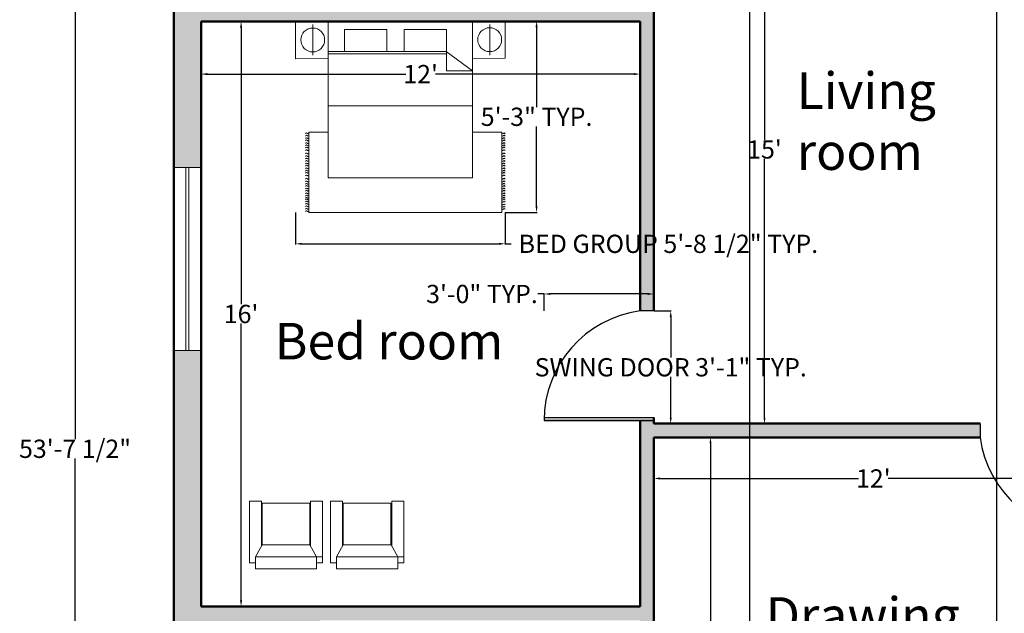
# Model space of a CAD drawing. Units: inches. Extents: x 2436 to 2989, y 5527 to 6207.
# Tile 2 of 5: x 2436 to 2759, y 5794 to 5989. Entities that reach past the tile are written whole.
import ezdxf

# ---------------------------------------------------------------- set-up
doc = ezdxf.new("R2010")
doc.units = ezdxf.units.IN
doc.header["$MEASUREMENT"] = 0
for name, color, linetype, lineweight in [('A-ANNO-DIMS', 2, 'Continuous', 18), ('A-AREA-IDEN', 7, 'Continuous', 25), ('A-DOOR', 3, 'Continuous', 25), ('A-FURN', 8, 'Continuous', 18), ('A-GLAZ', 4, 'Continuous', 18), ('A-WALL', 7, 'Continuous', 50), ('A-WALL-PATT', 252, 'Continuous', 13)]:
    doc.layers.add(name, color=color, linetype=linetype, lineweight=lineweight)
doc.styles.get("Standard").update_dxf_attribs({"font": 'arial.ttf'})
doc.dimstyles.get("Standard").update_dxf_attribs({"dimtxt": 6, "dimasz": 2, "dimexe": 0.18, "dimexo": 0.0625, "dimgap": 0.09, "dimtad": 0, "dimtih": 1, "dimtoh": 1, "dimdec": 0, "dimzin": 0, "dimdsep": 46, "dimlunit": 3, "dimtxsty": 'Standard', "dimcen": 0.09, "dimadec": 0, "dimazin": 0, "dimtfac": 1, "dimtdec": 0, "dimtofl": 0, "dimtmove": 0, "dimatfit": 3, "dimfxl": 1, "dimtolj": 1, "dimtzin": 0, "dimarcsym": 0})

# ---------------------------------------------------------------- blocks, each defined once
blk = doc.blocks.new('*D7')
at = {"layer": 'A-ANNO-DIMS', "color": 0, "lineweight": -2, "transparency": 16777216}
for p, q in [((2495.45, 5988.73), (2508.69, 5988.73)), ((2508.51, 5986.73), (2508.51, 5895.89)), ((2508.51, 5798.73), (2508.51, 5889.58)), ((2495.45, 5796.73), (2508.69, 5796.73))]:
    blk.add_line(p, q, dxfattribs=at)
at = {"layer": 'A-ANNO-DIMS', "color": 0, "transparency": 16777216}
for points in [[(2508.17, 5986.73), (2508.84, 5986.73), (2508.51, 5988.73)], [(2508.17, 5798.73), (2508.84, 5798.73), (2508.51, 5796.73)]]:
    blk.add_solid(points, dxfattribs=at)
at = {"layer": 'Defpoints', "color": 0, "transparency": 16777216}
for p in [(2495.39, 5988.73), (2495.39, 5796.73), (2508.51, 5796.73)]:
    blk.add_point(p, dxfattribs=at)
at = {"layer": 'A-ANNO-DIMS', "color": 0, "transparency": 16777216, "insert": (2508.51, 5892.73), "char_height": 6, "attachment_point": 5}
blk.add_mtext("\\A1;16'", dxfattribs=at)
blk = doc.blocks.new('*D8')
at = {"layer": 'A-ANNO-DIMS', "color": 0, "lineweight": -2, "transparency": 16777216}
for p, q in [((2495.39, 5988.67), (2495.39, 5971.26)), ((2639.39, 5988.67), (2639.39, 5971.26)), ((2497.39, 5971.44), (2562.49, 5971.44)), ((2637.39, 5971.44), (2572.29, 5971.44))]:
    blk.add_line(p, q, dxfattribs=at)
at = {"layer": 'A-ANNO-DIMS', "color": 0, "transparency": 16777216}
for points in [[(2497.39, 5971.78), (2497.39, 5971.11), (2495.39, 5971.44)], [(2637.39, 5971.78), (2637.39, 5971.11), (2639.39, 5971.44)]]:
    blk.add_solid(points, dxfattribs=at)
at = {"layer": 'Defpoints', "color": 0, "transparency": 16777216}
for p in [(2495.39, 5988.73), (2639.39, 5988.73), (2639.39, 5971.44)]:
    blk.add_point(p, dxfattribs=at)
at = {"layer": 'A-ANNO-DIMS', "color": 0, "transparency": 16777216, "insert": (2567.39, 5971.44), "char_height": 6, "attachment_point": 5}
blk.add_mtext("\\A1;12'", dxfattribs=at)
blk = doc.blocks.new('*D13')
at = {"layer": 'A-ANNO-DIMS', "color": 0, "lineweight": -2, "transparency": 16777216}
for p, q in [((2643.95, 5852.23), (2662.66, 5852.23)), ((2662.48, 5850.23), (2662.48, 5777.39)), ((2662.48, 5698.23), (2662.48, 5771.08)), ((2643.95, 5696.23), (2662.66, 5696.23))]:
    blk.add_line(p, q, dxfattribs=at)
at = {"layer": 'A-ANNO-DIMS', "color": 0, "transparency": 16777216}
for points in [[(2662.15, 5850.23), (2662.81, 5850.23), (2662.48, 5852.23)], [(2662.15, 5698.23), (2662.81, 5698.23), (2662.48, 5696.23)]]:
    blk.add_solid(points, dxfattribs=at)
at = {"layer": 'Defpoints', "color": 0, "transparency": 16777216}
for p in [(2643.89, 5852.23), (2643.89, 5696.23), (2662.48, 5696.23)]:
    blk.add_point(p, dxfattribs=at)
at = {"layer": 'A-ANNO-DIMS', "color": 0, "transparency": 16777216, "insert": (2662.48, 5774.23), "char_height": 6, "attachment_point": 5}
blk.add_mtext("\\A1;13'", dxfattribs=at)
blk = doc.blocks.new('*D14')
at = {"layer": 'A-ANNO-DIMS', "color": 0, "lineweight": -2, "transparency": 16777216}
for p, q in [((2643.89, 5852.17), (2643.89, 5838.55)), ((2787.89, 5852.17), (2787.89, 5838.55)), ((2645.89, 5838.73), (2710.99, 5838.73)), ((2785.89, 5838.73), (2720.79, 5838.73))]:
    blk.add_line(p, q, dxfattribs=at)
at = {"layer": 'A-ANNO-DIMS', "color": 0, "transparency": 16777216}
for points in [[(2645.89, 5839.07), (2645.89, 5838.4), (2643.89, 5838.73)], [(2785.89, 5839.07), (2785.89, 5838.4), (2787.89, 5838.73)]]:
    blk.add_solid(points, dxfattribs=at)
at = {"layer": 'Defpoints', "color": 0, "transparency": 16777216}
for p in [(2643.89, 5852.23), (2787.89, 5852.23), (2787.89, 5838.73)]:
    blk.add_point(p, dxfattribs=at)
at = {"layer": 'A-ANNO-DIMS', "color": 0, "transparency": 16777216, "insert": (2715.89, 5838.73), "char_height": 6, "attachment_point": 5}
blk.add_mtext("\\A1;12'", dxfattribs=at)
blk = doc.blocks.new('*D19')
at = {"layer": 'A-ANNO-DIMS', "color": 0, "lineweight": -2, "transparency": 16777216}
for p, q in [((2667.17, 6036.73), (2680.37, 6036.73)), ((2680.19, 6034.73), (2680.19, 5949.89)), ((2680.19, 5858.73), (2680.19, 5943.58)), ((2667.17, 5856.73), (2680.37, 5856.73))]:
    blk.add_line(p, q, dxfattribs=at)
at = {"layer": 'A-ANNO-DIMS', "color": 0, "transparency": 16777216}
for points in [[(2679.86, 6034.73), (2680.52, 6034.73), (2680.19, 6036.73)], [(2679.86, 5858.73), (2680.52, 5858.73), (2680.19, 5856.73)]]:
    blk.add_solid(points, dxfattribs=at)
at = {"layer": 'Defpoints', "color": 0, "transparency": 16777216}
for p in [(2667.11, 6036.73), (2667.11, 5856.73), (2680.19, 5856.73)]:
    blk.add_point(p, dxfattribs=at)
at = {"layer": 'A-ANNO-DIMS', "color": 0, "transparency": 16777216, "insert": (2680.19, 5946.73), "char_height": 6, "attachment_point": 5}
blk.add_mtext("\\A1;15'", dxfattribs=at)
blk = doc.blocks.new('BED-WITH-NIGHTSTANDS')
for p, q in [((5.6, 61.62), (5.6, 51.56)), ((63.65, 61.72), (63.65, 51.66)), ((49.39, 52.82), (10.63, 52.82)), ((49.44, 52), (10.63, 52)), ((49.39, 52.82), (58, 46.47)), ((49.44, 52.82), (49.44, 46.47)), ((49.44, 46.47), (58, 46.47)), ((58.05, 34.96), (10.63, 34.96)), ((4.35, 0), (4.35, 26.37)), ((4.35, 26.37), (10.65, 26.37)), ((58.05, 26.37), (67.59, 26.37)), ((67.59, 26.37), (67.59, 0)), ((4.35, 0), (67.59, 0))]:
    blk.add_line(p, q)
for points in [[(0, 50.39), (10.63, 50.5), (10.63, 62.68), (0, 62.58)], [(58.05, 62.68), (58.05, 11.37), (10.63, 11.37), (10.63, 62.68)], [(58.05, 50.5), (68.68, 50.6), (68.68, 62.78), (58.05, 62.68)], [(29.88, 59.98), (29.88, 52.82), (15.98, 52.82), (15.98, 59.98)], [(49.44, 59.98), (49.44, 52.82), (35.55, 52.82), (35.55, 59.98)]]:
    blk.add_lwpolyline(points, close=True)
for centre in [(5.6, 56.59), (63.65, 56.69)]:
    blk.add_circle(centre, 3.92)
for points, knots in [([(3.23, 25.84), (3.32, 25.96), (3.52, 26.2), (3.86, 25.96), (4.14, 25.78), (4.29, 25.89), (4.35, 25.94)], [0, 0, 0, 0, 0.400747, 0.791423, 1.067667, 1.29709, 1.29709, 1.29709, 1.29709]), ([(68.71, 25.84), (68.61, 25.96), (68.42, 26.2), (68.08, 25.96), (67.8, 25.78), (67.65, 25.89), (67.58, 25.94)], [0, 0, 0, 0, 0.400747, 0.791423, 1.067667, 1.29709, 1.29709, 1.29709, 1.29709]), ([(3.23, 25.06), (3.32, 25.18), (3.52, 25.42), (3.86, 25.18), (4.14, 25.01), (4.29, 25.11), (4.35, 25.16)], [0, 0, 0, 0, 0.400747, 0.791423, 1.067667, 1.29709, 1.29709, 1.29709, 1.29709]), ([(3.23, 24.24), (3.32, 24.36), (3.52, 24.6), (3.86, 24.36), (4.14, 24.19), (4.29, 24.3), (4.35, 24.34)], [0, 0, 0, 0, 0.400747, 0.791423, 1.067667, 1.29709, 1.29709, 1.29709, 1.29709]), ([(3.23, 23.51), (3.32, 23.63), (3.52, 23.87), (3.86, 23.63), (4.14, 23.46), (4.29, 23.57), (4.35, 23.62)], [0, 0, 0, 0, 0.400747, 0.791423, 1.067667, 1.29709, 1.29709, 1.29709, 1.29709]), ([(3.23, 22.63), (3.32, 22.75), (3.52, 22.99), (3.86, 22.75), (4.14, 22.58), (4.29, 22.69), (4.35, 22.73)], [0, 0, 0, 0, 0.400747, 0.791423, 1.067667, 1.29709, 1.29709, 1.29709, 1.29709]), ([(68.71, 25.06), (68.61, 25.18), (68.42, 25.42), (68.08, 25.18), (67.8, 25.01), (67.65, 25.11), (67.58, 25.16)], [0, 0, 0, 0, 0.400747, 0.791423, 1.067667, 1.29709, 1.29709, 1.29709, 1.29709]), ([(68.71, 24.24), (68.61, 24.36), (68.42, 24.6), (68.08, 24.36), (67.8, 24.19), (67.65, 24.3), (67.58, 24.34)], [0, 0, 0, 0, 0.400747, 0.791423, 1.067667, 1.29709, 1.29709, 1.29709, 1.29709]), ([(68.71, 23.51), (68.61, 23.63), (68.42, 23.87), (68.08, 23.63), (67.8, 23.46), (67.65, 23.57), (67.58, 23.62)], [0, 0, 0, 0, 0.400747, 0.791423, 1.067667, 1.29709, 1.29709, 1.29709, 1.29709]), ([(68.71, 22.63), (68.61, 22.75), (68.42, 22.99), (68.08, 22.75), (67.8, 22.58), (67.65, 22.69), (67.58, 22.73)], [0, 0, 0, 0, 0.400747, 0.791423, 1.067667, 1.29709, 1.29709, 1.29709, 1.29709]), ([(3.23, 21.88), (3.32, 22), (3.52, 22.24), (3.86, 22), (4.14, 21.83), (4.29, 21.93), (4.35, 21.98)], [0, 0, 0, 0, 0.400747, 0.791423, 1.067667, 1.29709, 1.29709, 1.29709, 1.29709]), ([(3.23, 21.15), (3.32, 21.27), (3.52, 21.51), (3.86, 21.27), (4.14, 21.1), (4.29, 21.21), (4.35, 21.25)], [0, 0, 0, 0, 0.400747, 0.791423, 1.067667, 1.29709, 1.29709, 1.29709, 1.29709]), ([(3.23, 20.27), (3.32, 20.39), (3.52, 20.63), (3.86, 20.39), (4.14, 20.22), (4.29, 20.32), (4.35, 20.37)], [0, 0, 0, 0, 0.400747, 0.791423, 1.067667, 1.29709, 1.29709, 1.29709, 1.29709]), ([(3.23, 19.23), (3.32, 19.35), (3.52, 19.59), (3.86, 19.35), (4.14, 19.18), (4.29, 19.29), (4.35, 19.33)], [0, 0, 0, 0, 0.400747, 0.791423, 1.067667, 1.29709, 1.29709, 1.29709, 1.29709]), ([(68.71, 21.88), (68.61, 22), (68.42, 22.24), (68.08, 22), (67.8, 21.83), (67.65, 21.93), (67.58, 21.98)], [0, 0, 0, 0, 0.400747, 0.791423, 1.067667, 1.29709, 1.29709, 1.29709, 1.29709]), ([(68.71, 21.15), (68.61, 21.27), (68.42, 21.51), (68.08, 21.27), (67.8, 21.1), (67.65, 21.21), (67.58, 21.25)], [0, 0, 0, 0, 0.400747, 0.791423, 1.067667, 1.29709, 1.29709, 1.29709, 1.29709]), ([(68.71, 20.27), (68.61, 20.39), (68.42, 20.63), (68.08, 20.39), (67.8, 20.22), (67.65, 20.32), (67.58, 20.37)], [0, 0, 0, 0, 0.400747, 0.791423, 1.067667, 1.29709, 1.29709, 1.29709, 1.29709]), ([(68.71, 19.23), (68.61, 19.35), (68.42, 19.59), (68.08, 19.35), (67.8, 19.18), (67.65, 19.29), (67.58, 19.33)], [0, 0, 0, 0, 0.400747, 0.791423, 1.067667, 1.29709, 1.29709, 1.29709, 1.29709]), ([(3.23, 18.35), (3.32, 18.47), (3.52, 18.71), (3.86, 18.47), (4.14, 18.3), (4.29, 18.4), (4.35, 18.45)], [0, 0, 0, 0, 0.400747, 0.791423, 1.067667, 1.29709, 1.29709, 1.29709, 1.29709]), ([(3.23, 17.53), (3.32, 17.65), (3.52, 17.89), (3.86, 17.65), (4.14, 17.48), (4.29, 17.59), (4.35, 17.64)], [0, 0, 0, 0, 0.400747, 0.791423, 1.067667, 1.29709, 1.29709, 1.29709, 1.29709]), ([(3.23, 16.76), (3.32, 16.88), (3.52, 17.12), (3.86, 16.88), (4.14, 16.71), (4.29, 16.81), (4.35, 16.86)], [0, 0, 0, 0, 0.400747, 0.791423, 1.067667, 1.29709, 1.29709, 1.29709, 1.29709]), ([(3.23, 15.94), (3.32, 16.06), (3.52, 16.3), (3.86, 16.06), (4.14, 15.89), (4.29, 16), (4.35, 16.04)], [0, 0, 0, 0, 0.400747, 0.791423, 1.067667, 1.29709, 1.29709, 1.29709, 1.29709]), ([(68.71, 18.35), (68.61, 18.47), (68.42, 18.71), (68.08, 18.47), (67.8, 18.3), (67.65, 18.4), (67.58, 18.45)], [0, 0, 0, 0, 0.400747, 0.791423, 1.067667, 1.29709, 1.29709, 1.29709, 1.29709]), ([(68.71, 17.53), (68.61, 17.65), (68.42, 17.89), (68.08, 17.65), (67.8, 17.48), (67.65, 17.59), (67.58, 17.64)], [0, 0, 0, 0, 0.400747, 0.791423, 1.067667, 1.29709, 1.29709, 1.29709, 1.29709]), ([(68.71, 16.76), (68.61, 16.88), (68.42, 17.12), (68.08, 16.88), (67.8, 16.71), (67.65, 16.81), (67.58, 16.86)], [0, 0, 0, 0, 0.400747, 0.791423, 1.067667, 1.29709, 1.29709, 1.29709, 1.29709]), ([(68.71, 15.94), (68.61, 16.06), (68.42, 16.3), (68.08, 16.06), (67.8, 15.89), (67.65, 16), (67.58, 16.04)], [0, 0, 0, 0, 0.400747, 0.791423, 1.067667, 1.29709, 1.29709, 1.29709, 1.29709]), ([(3.23, 15.21), (3.32, 15.33), (3.52, 15.57), (3.86, 15.33), (4.14, 15.16), (4.29, 15.27), (4.35, 15.32)], [0, 0, 0, 0, 0.400747, 0.791423, 1.067667, 1.29709, 1.29709, 1.29709, 1.29709]), ([(3.23, 14.33), (3.32, 14.45), (3.52, 14.69), (3.86, 14.45), (4.14, 14.28), (4.29, 14.39), (4.35, 14.43)], [0, 0, 0, 0, 0.400747, 0.791423, 1.067667, 1.29709, 1.29709, 1.29709, 1.29709]), ([(3.23, 13.58), (3.32, 13.7), (3.52, 13.94), (3.86, 13.7), (4.14, 13.53), (4.29, 13.63), (4.35, 13.68)], [0, 0, 0, 0, 0.400747, 0.791423, 1.067667, 1.29709, 1.29709, 1.29709, 1.29709]), ([(3.23, 12.85), (3.32, 12.97), (3.52, 13.21), (3.86, 12.97), (4.14, 12.8), (4.29, 12.9), (4.35, 12.95)], [0, 0, 0, 0, 0.400747, 0.791423, 1.067667, 1.29709, 1.29709, 1.29709, 1.29709]), ([(68.71, 15.21), (68.61, 15.33), (68.42, 15.57), (68.08, 15.33), (67.8, 15.16), (67.65, 15.27), (67.58, 15.32)], [0, 0, 0, 0, 0.400747, 0.791423, 1.067667, 1.29709, 1.29709, 1.29709, 1.29709]), ([(68.71, 14.33), (68.61, 14.45), (68.42, 14.69), (68.08, 14.45), (67.8, 14.28), (67.65, 14.39), (67.58, 14.43)], [0, 0, 0, 0, 0.400747, 0.791423, 1.067667, 1.29709, 1.29709, 1.29709, 1.29709]), ([(68.71, 13.58), (68.61, 13.7), (68.42, 13.94), (68.08, 13.7), (67.8, 13.53), (67.65, 13.63), (67.58, 13.68)], [0, 0, 0, 0, 0.400747, 0.791423, 1.067667, 1.29709, 1.29709, 1.29709, 1.29709]), ([(68.71, 12.85), (68.61, 12.97), (68.42, 13.21), (68.08, 12.97), (67.8, 12.8), (67.65, 12.9), (67.58, 12.95)], [0, 0, 0, 0, 0.400747, 0.791423, 1.067667, 1.29709, 1.29709, 1.29709, 1.29709]), ([(3.23, 11.97), (3.32, 12.09), (3.52, 12.33), (3.86, 12.09), (4.14, 11.92), (4.29, 12.02), (4.35, 12.07)], [0, 0, 0, 0, 0.400747, 0.791423, 1.067667, 1.29709, 1.29709, 1.29709, 1.29709]), ([(3.23, 10.93), (3.32, 11.05), (3.52, 11.29), (3.86, 11.05), (4.14, 10.88), (4.29, 10.99), (4.35, 11.03)], [0, 0, 0, 0, 0.400747, 0.791423, 1.067667, 1.29709, 1.29709, 1.29709, 1.29709]), ([(3.23, 10.05), (3.32, 10.17), (3.52, 10.41), (3.86, 10.17), (4.14, 10), (4.29, 10.1), (4.35, 10.15)], [0, 0, 0, 0, 0.400747, 0.791423, 1.067667, 1.29709, 1.29709, 1.29709, 1.29709]), ([(68.71, 11.97), (68.61, 12.09), (68.42, 12.33), (68.08, 12.09), (67.8, 11.92), (67.65, 12.02), (67.58, 12.07)], [0, 0, 0, 0, 0.400747, 0.791423, 1.067667, 1.29709, 1.29709, 1.29709, 1.29709]), ([(68.71, 10.93), (68.61, 11.05), (68.42, 11.29), (68.08, 11.05), (67.8, 10.88), (67.65, 10.99), (67.58, 11.03)], [0, 0, 0, 0, 0.400747, 0.791423, 1.067667, 1.29709, 1.29709, 1.29709, 1.29709]), ([(68.71, 10.05), (68.61, 10.17), (68.42, 10.41), (68.08, 10.17), (67.8, 10), (67.65, 10.1), (67.58, 10.15)], [0, 0, 0, 0, 0.400747, 0.791423, 1.067667, 1.29709, 1.29709, 1.29709, 1.29709]), ([(3.23, 9.23), (3.32, 9.35), (3.52, 9.59), (3.86, 9.35), (4.14, 9.18), (4.29, 9.29), (4.35, 9.34)], [0, 0, 0, 0, 0.400747, 0.791423, 1.067667, 1.29709, 1.29709, 1.29709, 1.29709]), ([(3.23, 8.54), (3.32, 8.66), (3.52, 8.9), (3.86, 8.66), (4.14, 8.49), (4.29, 8.6), (4.35, 8.65)], [0, 0, 0, 0, 0.400747, 0.791423, 1.067667, 1.29709, 1.29709, 1.29709, 1.29709]), ([(3.23, 7.73), (3.32, 7.85), (3.52, 8.09), (3.86, 7.85), (4.14, 7.68), (4.29, 7.78), (4.35, 7.83)], [0, 0, 0, 0, 0.400747, 0.791423, 1.067667, 1.29709, 1.29709, 1.29709, 1.29709]), ([(3.23, 7), (3.32, 7.12), (3.52, 7.36), (3.86, 7.12), (4.14, 6.95), (4.29, 7.05), (4.35, 7.1)], [0, 0, 0, 0, 0.400747, 0.791423, 1.067667, 1.29709, 1.29709, 1.29709, 1.29709]), ([(68.71, 9.23), (68.61, 9.35), (68.42, 9.59), (68.08, 9.35), (67.8, 9.18), (67.65, 9.29), (67.58, 9.34)], [0, 0, 0, 0, 0.400747, 0.791423, 1.067667, 1.29709, 1.29709, 1.29709, 1.29709]), ([(68.71, 8.54), (68.61, 8.66), (68.42, 8.9), (68.08, 8.66), (67.8, 8.49), (67.65, 8.6), (67.58, 8.65)], [0, 0, 0, 0, 0.400747, 0.791423, 1.067667, 1.29709, 1.29709, 1.29709, 1.29709]), ([(68.71, 7.73), (68.61, 7.85), (68.42, 8.09), (68.08, 7.85), (67.8, 7.68), (67.65, 7.78), (67.58, 7.83)], [0, 0, 0, 0, 0.400747, 0.791423, 1.067667, 1.29709, 1.29709, 1.29709, 1.29709]), ([(68.71, 7), (68.61, 7.12), (68.42, 7.36), (68.08, 7.12), (67.8, 6.95), (67.65, 7.05), (67.58, 7.1)], [0, 0, 0, 0, 0.400747, 0.791423, 1.067667, 1.29709, 1.29709, 1.29709, 1.29709]), ([(3.23, 6.12), (3.32, 6.24), (3.52, 6.48), (3.86, 6.24), (4.14, 6.07), (4.29, 6.17), (4.35, 6.22)], [0, 0, 0, 0, 0.400747, 0.791423, 1.067667, 1.29709, 1.29709, 1.29709, 1.29709]), ([(3.23, 5.36), (3.32, 5.49), (3.52, 5.73), (3.86, 5.49), (4.14, 5.31), (4.29, 5.42), (4.35, 5.47)], [0, 0, 0, 0, 0.400747, 0.791423, 1.067667, 1.29709, 1.29709, 1.29709, 1.29709]), ([(3.23, 4.64), (3.32, 4.76), (3.52, 5), (3.86, 4.76), (4.14, 4.59), (4.29, 4.69), (4.35, 4.74)], [0, 0, 0, 0, 0.400747, 0.791423, 1.067667, 1.29709, 1.29709, 1.29709, 1.29709]), ([(3.23, 4.13), (3.32, 4.25), (3.52, 4.49), (3.86, 4.25), (4.14, 4.08), (4.29, 4.18), (4.35, 4.23)], [0, 0, 0, 0, 0.400747, 0.791423, 1.067667, 1.29709, 1.29709, 1.29709, 1.29709]), ([(3.23, 3.44), (3.32, 3.56), (3.52, 3.8), (3.86, 3.56), (4.14, 3.39), (4.29, 3.49), (4.35, 3.54)], [0, 0, 0, 0, 0.400747, 0.791423, 1.067667, 1.29709, 1.29709, 1.29709, 1.29709]), ([(68.71, 6.12), (68.61, 6.24), (68.42, 6.48), (68.08, 6.24), (67.8, 6.07), (67.65, 6.17), (67.58, 6.22)], [0, 0, 0, 0, 0.400747, 0.791423, 1.067667, 1.29709, 1.29709, 1.29709, 1.29709]), ([(68.71, 5.36), (68.61, 5.49), (68.42, 5.73), (68.08, 5.49), (67.8, 5.31), (67.65, 5.42), (67.58, 5.47)], [0, 0, 0, 0, 0.400747, 0.791423, 1.067667, 1.29709, 1.29709, 1.29709, 1.29709]), ([(68.71, 4.64), (68.61, 4.76), (68.42, 5), (68.08, 4.76), (67.8, 4.59), (67.66, 4.69), (67.59, 4.73)], [0, 0, 0, 0, 0.400747, 0.791423, 1.067667, 1.283686, 1.283686, 1.283686, 1.283686]), ([(68.72, 4.07), (68.62, 4.19), (68.43, 4.43), (68.09, 4.19), (67.81, 4.01), (67.66, 4.12), (67.59, 4.17)], [0, 0, 0, 0, 0.400747, 0.791423, 1.067667, 1.29709, 1.29709, 1.29709, 1.29709]), ([(68.72, 3.34), (68.62, 3.46), (68.43, 3.7), (68.09, 3.46), (67.81, 3.29), (67.66, 3.39), (67.59, 3.44)], [0, 0, 0, 0, 0.400747, 0.791423, 1.067667, 1.29709, 1.29709, 1.29709, 1.29709]), ([(3.23, 2.67), (3.32, 2.79), (3.52, 3.03), (3.86, 2.79), (4.14, 2.62), (4.29, 2.73), (4.35, 2.78)], [0, 0, 0, 0, 0.400747, 0.791423, 1.067667, 1.29709, 1.29709, 1.29709, 1.29709]), ([(3.23, 1.86), (3.32, 1.98), (3.52, 2.22), (3.86, 1.98), (4.14, 1.81), (4.29, 1.92), (4.35, 1.97)], [0, 0, 0, 0, 0.400747, 0.791423, 1.067667, 1.29709, 1.29709, 1.29709, 1.29709]), ([(3.23, 1.05), (3.32, 1.17), (3.52, 1.41), (3.86, 1.17), (4.14, 1), (4.29, 1.11), (4.35, 1.15)], [0, 0, 0, 0, 0.400747, 0.791423, 1.067667, 1.29709, 1.29709, 1.29709, 1.29709]), ([(3.23, 0.28), (3.32, 0.4), (3.52, 0.64), (3.86, 0.4), (4.14, 0.22), (4.29, 0.33), (4.35, 0.38)], [0, 0, 0, 0, 0.400747, 0.791423, 1.067667, 1.29709, 1.29709, 1.29709, 1.29709]), ([(68.72, 2.46), (68.62, 2.58), (68.43, 2.82), (68.09, 2.58), (67.81, 2.4), (67.66, 2.51), (67.59, 2.56)], [0, 0, 0, 0, 0.400747, 0.791423, 1.067667, 1.29709, 1.29709, 1.29709, 1.29709]), ([(68.72, 1.7), (68.62, 1.82), (68.43, 2.06), (68.09, 1.82), (67.81, 1.65), (67.66, 1.76), (67.59, 1.81)], [0, 0, 0, 0, 0.400747, 0.791423, 1.067667, 1.29709, 1.29709, 1.29709, 1.29709]), ([(68.72, 0.98), (68.62, 1.1), (68.43, 1.34), (68.09, 1.1), (67.81, 0.93), (67.67, 1.03), (67.6, 1.07)], [0, 0, 0, 0, 0.400747, 0.791423, 1.067667, 1.283686, 1.283686, 1.283686, 1.283686])]:
    blk.add_open_spline(points, degree=3, knots=knots)
blk = doc.blocks.new('CHAIR-ARM')
for p, q in [((0, 1.96), (0, 22.23)), ((3.92, 22.23), (0, 22.23)), ((3.92, 7.54), (3.92, 22.23)), ((19.74, 21.58), (19.74, 7.85)), ((20.05, 7.41), (20.05, 22.23)), ((20.05, 22.23), (23.98, 22.23)), ((23.98, 1.96), (23.98, 22.23)), ((1.96, 3.92), (4.17, 7.85)), ((19.81, 7.85), (22.01, 3.92)), ((1.96, 3.92), (23.98, 3.92)), ((1.96, 3.92), (1.96, 0)), ((22.01, 3.92), (22.01, 0)), ((0, 1.96), (1.96, 1.96)), ((1.96, 0), (22.01, 0)), ((22.01, 1.96), (23.98, 1.96))]:
    blk.add_line(p, q)
blk.add_lwpolyline([(19.74, 21.58), (4.17, 21.58), (4.17, 7.85), (19.81, 7.85)])
blk = doc.blocks.new('WINDOW-60IN')
for p, q in [((0, 9), (0, 0)), ((60, 9), (0, 9)), ((60, 0), (60, 9)), ((60, 5), (0, 5)), ((0, 4), (60, 4)), ((0, 0), (60, 0))]:
    blk.add_line(p, q)
blk = doc.blocks.new('DOOR-SWING-36IN')
for p, q in [((1, 0), (1, 36)), ((1, 36), (1, 0)), ((2, 36), (2, 0)), ((37, 0), (37, 4.5)), ((0, 0), (1, 0)), ((1, 0), (2, 0))]:
    blk.add_line(p, q)
blk.add_arc((1, -0.32), 36.32, 7.6281, 90)
blk = doc.blocks.new('*D34')
at = {"layer": 'A-ANNO-DIMS', "color": 0, "lineweight": -2, "transparency": 16777216}
for p, q in [((2553.14, 6000.14), (2553.14, 5996.42)), ((2577.11, 6000.14), (2577.11, 5996.42)), ((2555.14, 5996.6), (2575.11, 5996.6)), ((2577.11, 5996.6), (2579.11, 5996.6))]:
    blk.add_line(p, q, dxfattribs=at)
at = {"layer": 'A-ANNO-DIMS', "color": 0, "transparency": 16777216}
for points in [[(2555.14, 5996.94), (2555.14, 5996.27), (2553.14, 5996.6)], [(2575.11, 5996.94), (2575.11, 5996.27), (2577.11, 5996.6)]]:
    blk.add_solid(points, dxfattribs=at)
at = {"layer": 'Defpoints', "color": 0, "transparency": 16777216}
for p in [(2553.14, 6000.2), (2577.11, 6000.2), (2577.11, 5996.6)]:
    blk.add_point(p, dxfattribs=at)
at = {"layer": 'A-ANNO-DIMS', "color": 0, "transparency": 16777216, "insert": (2621.18, 5996.6), "char_height": 6, "attachment_point": 5}
blk.add_mtext('\\A1;ARMCHAIR 2\'-0" TYP.', dxfattribs=at)
blk = doc.blocks.new('*D36')
at = {"layer": 'A-ANNO-DIMS', "color": 0, "lineweight": -2, "transparency": 16777216}
for p, q in [((2526.4, 5925.99), (2526.4, 5915.56)), ((2595.12, 5925.99), (2595.12, 5915.56)), ((2528.4, 5915.74), (2593.12, 5915.74)), ((2595.12, 5915.74), (2597.12, 5915.74))]:
    blk.add_line(p, q, dxfattribs=at)
at = {"layer": 'A-ANNO-DIMS', "color": 0, "transparency": 16777216}
for points in [[(2528.4, 5916.08), (2528.4, 5915.41), (2526.4, 5915.74)], [(2593.12, 5916.08), (2593.12, 5915.41), (2595.12, 5915.74)]]:
    blk.add_solid(points, dxfattribs=at)
at = {"layer": 'Defpoints', "color": 0, "transparency": 16777216}
for p in [(2526.4, 5926.05), (2595.12, 5926.05), (2595.12, 5915.74)]:
    blk.add_point(p, dxfattribs=at)
at = {"layer": 'A-ANNO-DIMS', "color": 0, "transparency": 16777216, "insert": (2648.67, 5915.74), "char_height": 6, "attachment_point": 5}
blk.add_mtext('\\A1;BED GROUP 5\'-8 1/2" TYP.', dxfattribs=at)
blk = doc.blocks.new('*D37')
at = {"layer": 'A-ANNO-DIMS', "color": 0, "lineweight": -2, "transparency": 16777216}
for p, q in [((2595.18, 5988.83), (2605.61, 5988.83)), ((2605.43, 5986.83), (2605.43, 5960.6)), ((2605.43, 5928.05), (2605.43, 5954.29)), ((2595.18, 5926.05), (2605.61, 5926.05))]:
    blk.add_line(p, q, dxfattribs=at)
at = {"layer": 'A-ANNO-DIMS', "color": 0, "transparency": 16777216}
for points in [[(2605.09, 5986.83), (2605.76, 5986.83), (2605.43, 5988.83)], [(2605.09, 5928.05), (2605.76, 5928.05), (2605.43, 5926.05)]]:
    blk.add_solid(points, dxfattribs=at)
at = {"layer": 'Defpoints', "color": 0, "transparency": 16777216}
for p in [(2595.12, 5988.83), (2605.43, 5988.83), (2595.12, 5926.05)]:
    blk.add_point(p, dxfattribs=at)
at = {"layer": 'A-ANNO-DIMS', "color": 0, "transparency": 16777216, "insert": (2605.43, 5957.44), "char_height": 6, "attachment_point": 5}
blk.add_mtext('\\A1;5\'-3" TYP.', dxfattribs=at)
blk = doc.blocks.new('*D40')
at = {"layer": 'A-ANNO-DIMS', "color": 0, "lineweight": -2, "transparency": 16777216}
for p, q in [((2643.95, 5893.73), (2649.62, 5893.73)), ((2649.44, 5891.73), (2649.44, 5878.43)), ((2649.44, 5858.73), (2649.44, 5872.04)), ((2643.95, 5856.73), (2649.62, 5856.73))]:
    blk.add_line(p, q, dxfattribs=at)
at = {"layer": 'A-ANNO-DIMS', "color": 0, "transparency": 16777216}
for points in [[(2649.1, 5891.73), (2649.77, 5891.73), (2649.44, 5893.73)], [(2649.1, 5858.73), (2649.77, 5858.73), (2649.44, 5856.73)]]:
    blk.add_solid(points, dxfattribs=at)
at = {"layer": 'Defpoints', "color": 0, "transparency": 16777216}
for p in [(2643.89, 5893.73), (2649.44, 5893.73), (2643.89, 5856.73)]:
    blk.add_point(p, dxfattribs=at)
at = {"layer": 'A-ANNO-DIMS', "color": 0, "transparency": 16777216, "insert": (2649.44, 5875.23), "char_height": 6, "attachment_point": 5}
blk.add_mtext('\\A1;SWING DOOR 3\'-1" TYP.', dxfattribs=at)
blk = doc.blocks.new('*D41')
at = {"layer": 'A-ANNO-DIMS', "color": 0, "lineweight": -2, "transparency": 16777216}
for p, q in [((2607.89, 5899.28), (2605.89, 5899.28)), ((2607.89, 5893.79), (2607.89, 5899.46)), ((2641.89, 5899.28), (2609.89, 5899.28)), ((2643.89, 5893.79), (2643.89, 5899.46))]:
    blk.add_line(p, q, dxfattribs=at)
at = {"layer": 'A-ANNO-DIMS', "color": 0, "transparency": 16777216}
for points in [[(2609.89, 5899.62), (2609.89, 5898.95), (2607.89, 5899.28)], [(2641.89, 5899.62), (2641.89, 5898.95), (2643.89, 5899.28)]]:
    blk.add_solid(points, dxfattribs=at)
at = {"layer": 'Defpoints', "color": 0, "transparency": 16777216}
for p in [(2607.89, 5899.28), (2607.89, 5893.73), (2643.89, 5893.73)]:
    blk.add_point(p, dxfattribs=at)
at = {"layer": 'A-ANNO-DIMS', "color": 0, "transparency": 16777216, "insert": (2587.51, 5899.28), "char_height": 6, "attachment_point": 5}
blk.add_mtext('\\A1;3\'-0" TYP.', dxfattribs=at)
blk = doc.blocks.new('*D49')
at = {"layer": 'A-ANNO-DIMS', "color": 0, "lineweight": -2, "transparency": 16777216}
for p, q in [((2486.33, 6170.23), (2453.86, 6170.23)), ((2454.04, 6168.23), (2454.04, 5851.68)), ((2454.04, 5528.73), (2454.04, 5845.29)), ((2675.33, 5526.73), (2453.86, 5526.73))]:
    blk.add_line(p, q, dxfattribs=at)
at = {"layer": 'A-ANNO-DIMS', "color": 0, "transparency": 16777216}
for points in [[(2453.7, 6168.23), (2454.37, 6168.23), (2454.04, 6170.23)], [(2453.7, 5528.73), (2454.37, 5528.73), (2454.04, 5526.73)]]:
    blk.add_solid(points, dxfattribs=at)
at = {"layer": 'Defpoints', "color": 0, "transparency": 16777216}
for p in [(2486.39, 6170.23), (2454.04, 5526.73), (2675.39, 5526.73)]:
    blk.add_point(p, dxfattribs=at)
at = {"layer": 'A-ANNO-DIMS', "color": 0, "transparency": 16777216, "insert": (2454.04, 5848.48), "char_height": 6, "attachment_point": 5}
blk.add_mtext('\\A1;53\'-7 1/2"', dxfattribs=at)
blk = doc.blocks.new('*D51')
at = {"layer": 'A-ANNO-DIMS', "color": 0, "lineweight": -2, "transparency": 16777216}
for p, q in [((2675.39, 5526.79), (2675.39, 6202.76)), ((2677.39, 6202.58), (2707.81, 6202.58)), ((2754.39, 6202.58), (2723.97, 6202.58)), ((2756.39, 5526.79), (2756.39, 6202.76))]:
    blk.add_line(p, q, dxfattribs=at)
at = {"layer": 'A-ANNO-DIMS', "color": 0, "transparency": 16777216}
for points in [[(2677.39, 6202.92), (2677.39, 6202.25), (2675.39, 6202.58)], [(2754.39, 6202.92), (2754.39, 6202.25), (2756.39, 6202.58)]]:
    blk.add_solid(points, dxfattribs=at)
at = {"layer": 'Defpoints', "color": 0, "transparency": 16777216}
for p in [(2756.39, 6202.58), (2675.39, 5526.73), (2756.39, 5526.73)]:
    blk.add_point(p, dxfattribs=at)
at = {"layer": 'A-ANNO-DIMS', "color": 0, "transparency": 16777216, "insert": (2715.89, 6202.58), "char_height": 6, "attachment_point": 5}
blk.add_mtext('\\A1;6\'-9"', dxfattribs=at)
blk = doc.blocks.new('*D54')
at = {"layer": 'A-ANNO-DIMS', "color": 0, "lineweight": -2, "transparency": 16777216}
for p, q in [((2638.98, 6035.73), (2639.16, 6035.73)), ((2639.07, 6035.64), (2639.07, 6035.82)), ((2682.8, 5997.46), (2667.91, 6010.5)), ((2684.8, 5997.46), (2682.8, 5997.46))]:
    blk.add_line(p, q, dxfattribs=at)
at = {"layer": 'A-ANNO-DIMS', "color": 0, "transparency": 16777216}
blk.add_solid([(2668.13, 6010.75), (2667.69, 6010.25), (2666.4, 6011.81)], dxfattribs=at)
at = {"layer": 'Defpoints', "color": 0, "transparency": 16777216}
for p in [(2639.07, 6035.73), (2666.4, 6011.81)]:
    blk.add_point(p, dxfattribs=at)
at = {"layer": 'A-ANNO-DIMS', "color": 0, "transparency": 16777216, "insert": (2709.19, 5997.46), "char_height": 6, "attachment_point": 5}
blk.add_mtext('\\A1;6X R3\'-0 1/2"', dxfattribs=at)

msp = doc.modelspace()

# ---------------------------------------------------------------- hatches: boundary and pattern name
at = {"layer": 'A-WALL-PATT'}
h = msp.add_hatch(color=256, dxfattribs=at)
h.dxf.hatch_style = 1
h.paths.add_polyline_path([(2533.49, 6170.23), (2486.39, 6170.23), (2486.39, 6124.33), (2495.39, 6124.33), (2495.39, 6161.23), (2533.49, 6161.23)])
h.paths.add_polyline_path([(2677.58, 6170.23), (2593.49, 6170.23), (2593.49, 6161.23), (2639.39, 6161.23), (2639.39, 6035.73), (2639.39, 6035.73), (2643.89, 6035.73), (2643.89, 6036.73), (2685.89, 6036.73), (2685.89, 6041.23), (2643.89, 6041.23), (2643.89, 6161.23), (2677.58, 6161.23)])
h.paths.add_polyline_path([(2792.39, 6170.23), (2737.58, 6170.23), (2737.58, 6161.23), (2787.89, 6161.23), (2787.89, 6084.23), (2792.39, 6084.23), (2792.39, 6161.23), (2936.39, 6161.23), (2936.39, 6071.23), (2840.39, 6071.23), (2840.39, 6047.23), (2792.39, 6047.23), (2792.39, 6048.23), (2787.89, 6048.23), (2787.89, 6047.23), (2787.89, 6041.23), (2742.3, 6041.23), (2742.3, 6036.73), (2787.89, 6036.73), (2787.89, 6035.73), (2792.39, 6035.73), (2792.39, 6042.73), (2840.39, 6042.73), (2840.39, 5945.23), (2792.39, 5945.23), (2792.39, 6003.73), (2787.89, 6003.73), (2787.89, 5893.73), (2792.39, 5893.73), (2792.39, 5940.73), (2845.89, 5940.73), (2845.89, 5945.23), (2844.89, 5945.23), (2844.89, 6047.23), (2844.89, 6066.73), (2936.39, 6066.73), (2936.39, 6024.33), (2945.39, 6024.33), (2945.39, 6080.66), (2940.89, 6080.66), (2940.89, 6165.73), (2792.39, 6165.73)])
h.paths.add_polyline_path([(2945.39, 6000.33), (2936.39, 6000.33), (2936.39, 5945.23), (2881.89, 5945.23), (2881.89, 5940.73), (2936.39, 5940.73), (2936.39, 5901.74), (2945.39, 5901.74)], flags=17)
h.paths.add_polyline_path([(2945.39, 5841.74), (2936.39, 5841.74), (2936.39, 5796.73), (2792.39, 5796.73), (2792.39, 5857.73), (2787.89, 5857.73), (2787.89, 5856.73), (2786.89, 5856.73), (2786.89, 5852.23), (2787.89, 5852.23), (2787.89, 5792.23), (2892.89, 5792.23), (2892.89, 5760.78), (2901.89, 5760.78), (2901.89, 5792.23), (2945.39, 5792.23)])
h.paths.add_polyline_path([(2495.39, 5880.74), (2486.39, 5880.74), (2486.39, 5787.73), (2525.39, 5787.73), (2525.39, 5761.57), (2534.39, 5761.57), (2534.39, 5792.23), (2639.39, 5792.23), (2639.39, 5733.23), (2643.89, 5733.23), (2643.89, 5852.23), (2750.89, 5852.23), (2750.89, 5856.73), (2643.89, 5856.73), (2643.89, 5857.73), (2639.39, 5857.73), (2639.39, 5796.73), (2495.39, 5796.73)])
h.paths.add_polyline_path([(2495.39, 6064.33), (2486.39, 6064.33), (2486.39, 5940.74), (2495.39, 5940.74), (2495.39, 5988.73), (2639.39, 5988.73), (2639.39, 5893.73), (2643.89, 5893.73), (2643.89, 5999.73), (2639.39, 5999.73), (2639.39, 5993.23), (2495.39, 5993.23)])
h.paths.add_polyline_path([(2682.14, 5696.23), (2643.89, 5696.23), (2643.89, 5697.23), (2639.39, 5697.23), (2639.39, 5696.23), (2558.39, 5696.23), (2534.39, 5696.23), (2534.39, 5737.57), (2525.39, 5737.57), (2525.39, 5687.23), (2534.39, 5687.23), (2558.39, 5687.23), (2643.89, 5687.23), (2682.14, 5687.23)])
h.paths.add_polyline_path([(2901.89, 5736.78), (2892.89, 5736.78), (2892.89, 5696.23), (2868.89, 5696.23), (2751.89, 5696.23), (2751.89, 5687.23), (2787.89, 5687.23), (2787.89, 5567.23), (2792.39, 5567.23), (2792.39, 5687.23), (2868.89, 5687.23), (2892.89, 5687.23), (2901.89, 5687.23)])
h.paths.add_polyline_path([(2643.89, 5687.23), (2639.39, 5687.23), (2639.39, 5567.23), (2643.89, 5567.23)])
h.paths.add_polyline_path([(2787.89, 5567.23), (2643.89, 5567.23), (2643.89, 5562.73), (2787.89, 5562.73)])
h.paths.add_polyline_path([(2643.89, 5567.23), (2639.39, 5567.23), (2639.39, 5562.73), (2643.89, 5562.73)])
h.paths.add_polyline_path([(2792.39, 5567.23), (2787.89, 5567.23), (2787.89, 5562.73), (2792.39, 5562.73)])

# ---------------------------------------------------------------- linework, layer by layer
at = {"layer": 'A-DOOR'}
msp.add_line((2643.89, 5857.73), (2643.89, 5857.73), dxfattribs=at)
at = {"layer": 'A-WALL'}
for p, q in [((2486.39, 6170.23), (2486.39, 5787.73)), ((2643.89, 5999.73), (2643.89, 5893.73)), ((2495.39, 5988.73), (2639.39, 5988.73)), ((2495.39, 5988.73), (2495.39, 5796.73)), ((2639.39, 5988.73), (2639.39, 5893.73)), ((2639.39, 5857.73), (2639.39, 5796.73)), ((2643.89, 5858.73), (2643.89, 5856.73)), ((2643.89, 5856.73), (2750.89, 5856.73)), ((2643.89, 5852.23), (2750.89, 5852.23)), ((2643.89, 5852.23), (2643.89, 5733.23)), ((2495.39, 5796.73), (2639.39, 5796.73))]:
    msp.add_line(p, q, dxfattribs=at)

# ---------------------------------------------------------------- block references
at = {"layer": 'A-DOOR'}
for p, rotation in [((2643.89, 5856.73), 89.99999999999706), ((2787.89, 5856.73), 180)]:
    msp.add_blockref('DOOR-SWING-36IN', p, dxfattribs=dict(at, rotation=rotation))
at = {"layer": 'A-FURN'}
for name, p in [('BED-WITH-NIGHTSTANDS', (2526.4, 5926.05)), ('CHAIR-ARM', (2511.26, 5809.1)), ('CHAIR-ARM', (2537.87, 5809.1))]:
    msp.add_blockref(name, p, dxfattribs=at)
at = {"layer": 'A-GLAZ', "rotation": 270.0000000000035}
msp.add_blockref('WINDOW-60IN', (2486.39, 5940.74), dxfattribs=at)

# ---------------------------------------------------------------- texts
at = {"layer": 'A-AREA-IDEN', "char_height": 12, "attachment_point": 1}
for s, width, insert in [('Living\\Proom', 82.618, (2690.77, 5972)), ('Bed room', 77.0308, (2519.53, 5889.8)), ('Drawing\\Proom', 69.5872, (2680.57, 5799.76))]:
    msp.add_mtext_dynamic_manual_height_columns(s, width=width, gutter_width=1, heights=[0], dxfattribs=dict(at, insert=insert))

# ---------------------------------------------------------------- dimensions: what is measured, and where the dimension line sits
at = {"layer": 'A-ANNO-DIMS'}
for base, p1, p2, override, picture, middle in [((2756.39, 6202.58), (2675.39, 5526.73), (2756.39, 5526.73), {"dimdec": 1, "dimlfac": 1, "dimrnd": 0, "dimzin": 1, "dimdsep": 46, "dimlunit": 4, "dimfrac": 2}, '*D51', (2715.89, 6202.58)), ((2639.39, 5971.44), (2495.39, 5988.73), (2639.39, 5988.73), {"dimclrd": 0, "dimclre": 0, "dimclrt": 0}, '*D8', (2567.39, 5971.44)), ((2787.89, 5838.73), (2643.89, 5852.23), (2787.89, 5852.23), {"dimclrd": 0, "dimclre": 0, "dimclrt": 0}, '*D14', (2715.89, 5838.73))]:
    dim = msp.add_linear_dim(base=base, p1=p1, p2=p2, dimstyle='Standard', override=override, dxfattribs=at)
    dim.commit()
    dim.dimension.update_dxf_attribs({"geometry": picture, "text_midpoint": middle})
for base, p1, p2, override, picture, middle in [((2454.04, 5526.73), (2486.39, 6170.23), (2675.39, 5526.73), {"dimdec": 1, "dimlfac": 1, "dimrnd": 0, "dimzin": 1, "dimdsep": 46, "dimlunit": 4, "dimfrac": 2}, '*D49', (2454.04, 5848.48)), ((2680.19, 5856.73), (2667.11, 6036.73), (2667.11, 5856.73), {"dimclrd": 0, "dimclre": 0, "dimclrt": 0}, '*D19', (2680.19, 5946.73)), ((2508.51, 5796.73), (2495.39, 5988.73), (2495.39, 5796.73), {"dimclrd": 0, "dimclre": 0, "dimclrt": 0}, '*D7', (2508.51, 5892.73)), ((2662.48, 5696.23), (2643.89, 5852.23), (2643.89, 5696.23), {"dimclrd": 0, "dimclre": 0, "dimclrt": 0}, '*D13', (2662.48, 5774.23))]:
    dim = msp.add_linear_dim(base=base, p1=p1, p2=p2, angle=90, dimstyle='Standard', override=override, dxfattribs=at)
    dim.commit()
    dim.dimension.update_dxf_attribs({"geometry": picture, "text_midpoint": middle})
dim = msp.add_radius_dim(center=(2639.07, 6035.73), mpoint=(2666.4, 6011.81), text='6X <>', dimstyle='Standard', override={"dimdec": 1, "dimlfac": 1, "dimrnd": 0, "dimzin": 1, "dimdsep": 46, "dimlunit": 4, "dimfrac": 2}, dxfattribs=at)
dim.commit()
dim.dimension.update_dxf_attribs({"geometry": '*D54', "text_midpoint": (2709.19, 5997.46), "dimtype": 164})
for base, p1, p2, text, picture, middle in [((2577.11, 5996.6), (2553.14, 6000.2), (2577.11, 6000.2), 'ARMCHAIR <> TYP.', '*D34', (2621.18, 5996.6)), ((2595.12, 5915.74), (2526.4, 5926.05), (2595.12, 5926.05), 'BED GROUP <> TYP.', '*D36', (2648.67, 5915.74))]:
    dim = msp.add_linear_dim(base=base, p1=p1, p2=p2, text=text, dimstyle='Standard', override={"dimdec": 1, "dimlfac": 1, "dimrnd": 0, "dimzin": 1, "dimdsep": 46, "dimlunit": 4, "dimfrac": 2}, dxfattribs=at)
    dim.commit()
    dim.dimension.update_dxf_attribs({"geometry": picture, "text_midpoint": middle})
for base, p1, p2, angle, text, picture, middle in [((2605.43, 5988.83), (2595.12, 5926.05), (2595.12, 5988.83), 90, '<> TYP.', '*D37', (2605.43, 5957.44)), ((2607.89, 5899.28), (2643.89, 5893.73), (2607.89, 5893.73), 180, '<> TYP.', '*D41', (2587.51, 5899.28)), ((2649.44, 5893.73), (2643.89, 5856.73), (2643.89, 5893.73), 90, 'SWING DOOR <> TYP.', '*D40', (2649.44, 5875.23))]:
    dim = msp.add_linear_dim(base=base, p1=p1, p2=p2, angle=angle, text=text, dimstyle='Standard', override={"dimdec": 1, "dimlfac": 1, "dimrnd": 0, "dimzin": 1, "dimdsep": 46, "dimlunit": 4, "dimfrac": 2}, dxfattribs=at)
    dim.commit()
    dim.dimension.update_dxf_attribs({"geometry": picture, "text_midpoint": middle})

doc.saveas('drawing.dxf')
